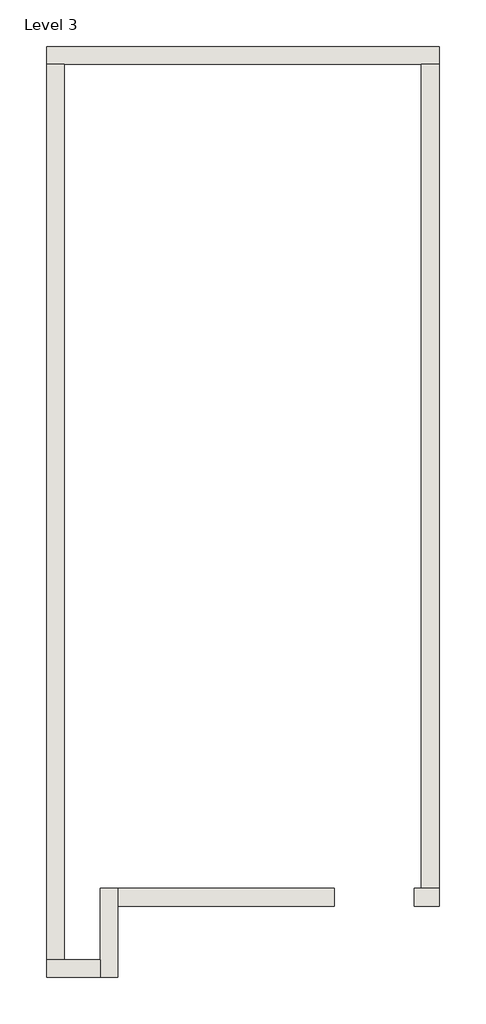
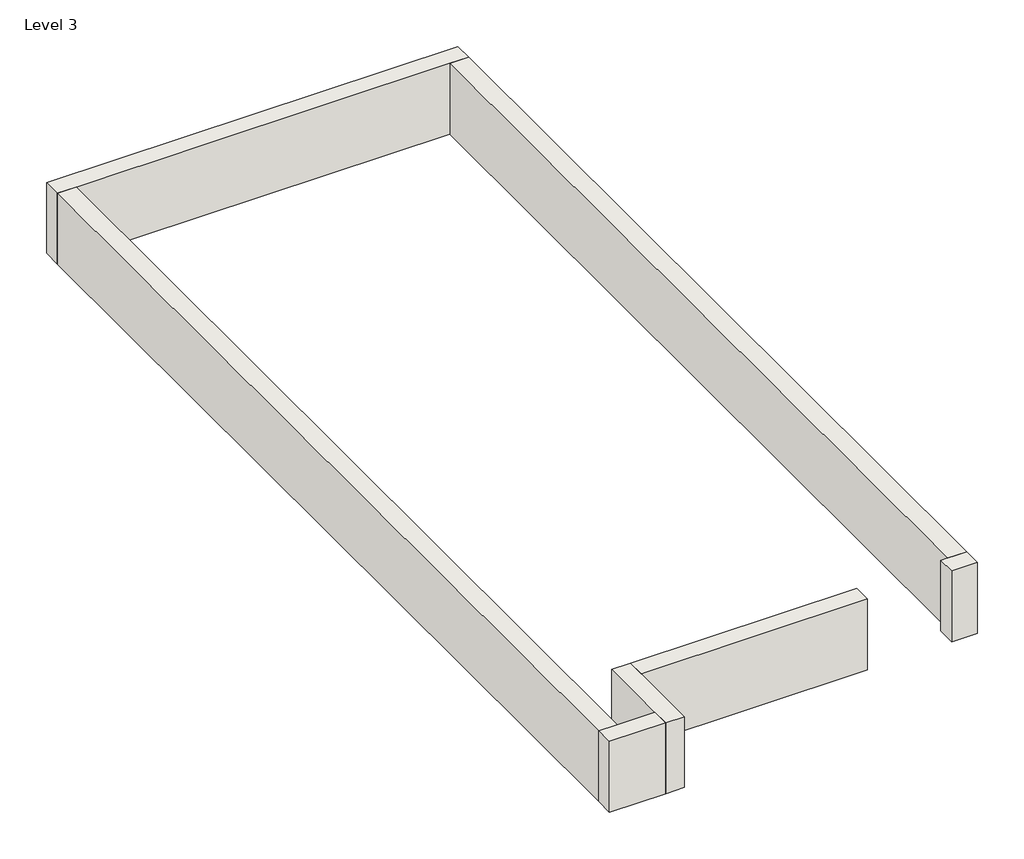
# One storey: 7 walls.
"""IFC4 building model written with IfcOpenShell, lengths in millimetres."""

from ifc_helpers import new_model, si_unit, frame, origin, place, context, project, spatial, polyline, outline, extrude, faceted_brep, element, save

model = new_model("IFC4")

# Units and contexts
model_context = context("Model", 3, world=origin())
ifc_project = project(units=[si_unit("LENGTHUNIT", "METRE", prefix="MILLI")], contexts=[model_context])

# Site, building, storey
site = spatial("IfcSite", under=ifc_project)
building = spatial("IfcBuilding", under=site)
storey = spatial("IfcBuildingStorey", under=building, Name="Level 3", Elevation=6096.0)

# Walls
placement = place(None, origin())
element("IfcWall", 1, ObjectType="wall 9\"", at=placement, inside=storey, context=model_context, shape_type="Brep", body=[
    faceted_brep([(-5651.4766939, 2068.0902438, 6096.0), (-5422.8766939, 2068.0902438, 6096.0), (-850.8766939, 2068.0902438, 6096.0), (-622.2766939, 2068.0902438, 6096.0), (-622.2766939, 2068.0902438, 7010.4), (-850.8766939, 2068.0902438, 7010.4), (-5422.8766939, 2068.0902438, 7010.4), (-5651.4766939, 2068.0902438, 7010.4), (-5651.4766939, 2296.6902438, 6096.0), (-5651.4766939, 2296.6902438, 7010.4), (-622.2766939, 2296.6902438, 7010.4), (-622.2766939, 2296.6902438, 6096.0)], [[[0, 1, 2, 3, 4, 5, 6, 7]], [[8, 9, 10, 11]], [[3, 2, 1, 0, 8, 11]], [[7, 6, 5, 4, 10, 9]], [[4, 3, 11, 10]], [[0, 7, 9, 8]]]),
])
element("IfcWall", 2, ObjectType="wall 9\"", at=placement, inside=storey, context=model_context, shape_type="SweptSolid", body=[
    extrude(outline(polyline([(-850.8766939, -8485.6097562), (-850.8766939, 2068.0902438), (-622.2766939, 2068.0902438), (-622.2766939, -8485.6097562), (-850.8766939, -8485.6097562)])), frame((0.0, 0.0, 6096.0), z_axis=(0.0, 0.0, 1.0), x_axis=(1.0, 0.0, 0.0)), (0.0, 0.0, 1.0), 914.4),
])
element("IfcWall", 3, ObjectType="wall 9\"", at=placement, inside=storey, context=model_context, shape_type="Brep", body=[
    faceted_brep([(-4965.6766939, -8485.6097562, 6096.0), (-4965.6766939, -9400.0097562, 6096.0), (-4965.6766939, -9628.6097562, 6096.0), (-4965.6766939, -9628.6097562, 7010.4), (-4965.6766939, -9400.0097562, 7010.4), (-4965.6766939, -8485.6097562, 7010.4), (-4737.0766939, -8485.6097562, 6096.0), (-4737.0766939, -8485.6097562, 7010.4), (-4737.0766939, -8714.2097562, 7010.4), (-4737.0766939, -9628.6097562, 7010.4), (-4737.0766939, -9628.6097562, 6096.0), (-4737.0766939, -8714.2097562, 6096.0)], [[[0, 1, 2, 3, 4, 5]], [[6, 7, 8, 9, 10, 11]], [[2, 1, 0, 6, 11, 10]], [[5, 4, 3, 9, 8, 7]], [[3, 2, 10, 9]], [[0, 5, 7, 6]]]),
])
element("IfcWall", 4, ObjectType="wall 9\"", at=placement, inside=storey, context=model_context, shape_type="Brep", body=[
    faceted_brep([(-4965.6766939, -9400.0097562, 6096.0), (-5422.8766939, -9400.0097562, 6096.0), (-5651.4766939, -9400.0097562, 6096.0), (-5651.4766939, -9400.0097562, 7010.4), (-5422.8766939, -9400.0097562, 7010.4), (-4965.6766939, -9400.0097562, 7010.4), (-4965.6766939, -9628.6097562, 6096.0), (-4965.6766939, -9628.6097562, 7010.4), (-5651.4766939, -9628.6097562, 7010.4), (-5651.4766939, -9628.6097562, 6096.0)], [[[0, 1, 2, 3, 4, 5]], [[6, 7, 8, 9]], [[2, 1, 0, 6, 9]], [[5, 4, 3, 8, 7]], [[0, 5, 7, 6]], [[3, 2, 9, 8]]]),
])
element("IfcWall", 5, ObjectType="wall 9\"", at=placement, inside=storey, context=model_context, shape_type="SweptSolid", body=[
    extrude(outline(polyline([(-5422.8766939, 2068.0902438), (-5422.8766939, -9400.0097562), (-5651.4766939, -9400.0097562), (-5651.4766939, 2068.0902438), (-5422.8766939, 2068.0902438)])), frame((0.0, 0.0, 6096.0), z_axis=(0.0, 0.0, 1.0), x_axis=(1.0, 0.0, 0.0)), (0.0, 0.0, 1.0), 914.4),
])
element("IfcWall", 6, ObjectType="wall 9\"", at=placement, inside=storey, context=model_context, shape_type="SweptSolid", body=[
    extrude(outline(polyline([(-1968.4766939, -8714.2097562), (-4737.0766939, -8714.2097562), (-4737.0766939, -8485.6097562), (-1968.4766939, -8485.6097562), (-1968.4766939, -8714.2097562)])), frame((0.0, 0.0, 6096.0), z_axis=(0.0, 0.0, 1.0), x_axis=(1.0, 0.0, 0.0)), (0.0, 0.0, 1.0), 914.4),
])
element("IfcWall", 7, ObjectType="wall 9\"", at=placement, inside=storey, context=model_context, shape_type="Brep", body=[
    faceted_brep([(-622.2766939, -8485.6097562, 6096.0), (-850.8766939, -8485.6097562, 6096.0), (-938.0563134, -8485.6097562, 6096.0), (-938.0563134, -8485.6097562, 7010.4), (-850.8766939, -8485.6097562, 7010.4), (-622.2766939, -8485.6097562, 7010.4), (-622.2766939, -8714.2097562, 6096.0), (-622.2766939, -8714.2097562, 7010.4), (-938.0563134, -8714.2097562, 7010.4), (-938.0563134, -8714.2097562, 6096.0)], [[[0, 1, 2, 3, 4, 5]], [[6, 7, 8, 9]], [[2, 1, 0, 6, 9]], [[3, 2, 9, 8]], [[5, 4, 3, 8, 7]], [[0, 5, 7, 6]]]),
])

save(model, "model.ifc")

# Revit data of these elements
# Type "wall 9\""
#   Assembly Code = "B2010"
#   Layers, outside or top first: 0' - 9" no material (function 1)
# Elements 1, 2, 3, 4, 5, 6, 7 (IfcWall, "wall 9\"")
#   Top Offset = 0' - 0"
#   Base Offset = 0' - 0"
#   wall height = 3' - 0"
#   Phase Created = New Construction
#   Base Constraint = Level 3
#   Top Constraint = Level 6
#   Materials on its faces: "Default Wall"
# Materials
#   "Default Wall": colour RGB 128 128 128, transparency 0, Cost = 0
